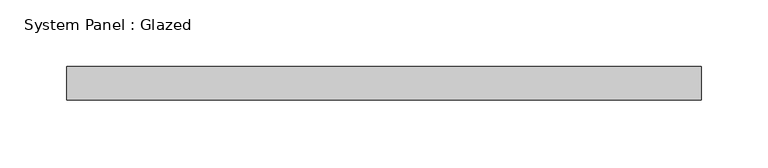
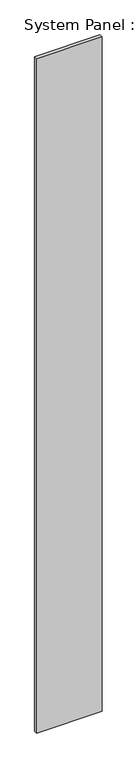
"""IFC4 building model written with IfcOpenShell, lengths in millimetres: plate geometry, System Panel : Glazed."""

from ifc_helpers import new_model, si_unit, origin, origin_with_axes, place, context, project, spatial, polyline, outline, extrude, source, transform, mapped, element, save


def system_panel_glazed_aa365302(model_context):
    return source(origin(), model_context, "Body", "SweptSolid", [
        extrude(outline(polyline([(238.324156, 19.05), (-238.324156, 19.05), (-238.324156, 44.45), (238.324156, 44.45), (238.324156, 19.05)])), origin_with_axes(), (0.0, 0.0, 1.0), 5190.545847),
    ])


if __name__ == "__main__":
    model = new_model("IFC4")
    model_context = context("Model", 3, world=origin())
    ifc_project = project(units=[si_unit("LENGTHUNIT", "METRE", prefix="MILLI")], contexts=[model_context])
    site = spatial("IfcSite", under=ifc_project)
    building = spatial("IfcBuilding", under=site)
    placement = place(None, origin())
    system_panel_glazed_shape = system_panel_glazed_aa365302(model_context)
    element("IfcPlate", 1, ObjectType="System Panel : Glazed", at=placement, inside=building, context=model_context, shape_type="MappedRepresentation", body=[
        mapped(system_panel_glazed_shape, transform((0.0, 0.0, 0.0), x_axis=(1.0, 0.0, 0.0), y_axis=(0.0, 1.0, 0.0), z_axis=(0.0, 0.0, 1.0))),
    ])
    save(model, "model.ifc")

# Revit data of these elements
# Type "System Panel : Glazed"
#   Construction Type Id = "GSP4R"
#   Analytic Construction = "1/8 in Pilkington single glazing"
#   Visual Light Transmittance = 0.9
#   Solar Heat Gain Coefficient = 0.86
#   Heat Transfer Coefficient (U) = 1.18115 BTU/(h·ft²·°F)
# Element 1 (IfcPlate, "System Panel : Glazed")
#   Materials on its faces: "Glass"
# Materials
#   "Glass": class "Glass", colour RGB 0 128 192, transparency 0.75, Description = "Soda Lime Glass", Cost = 0
